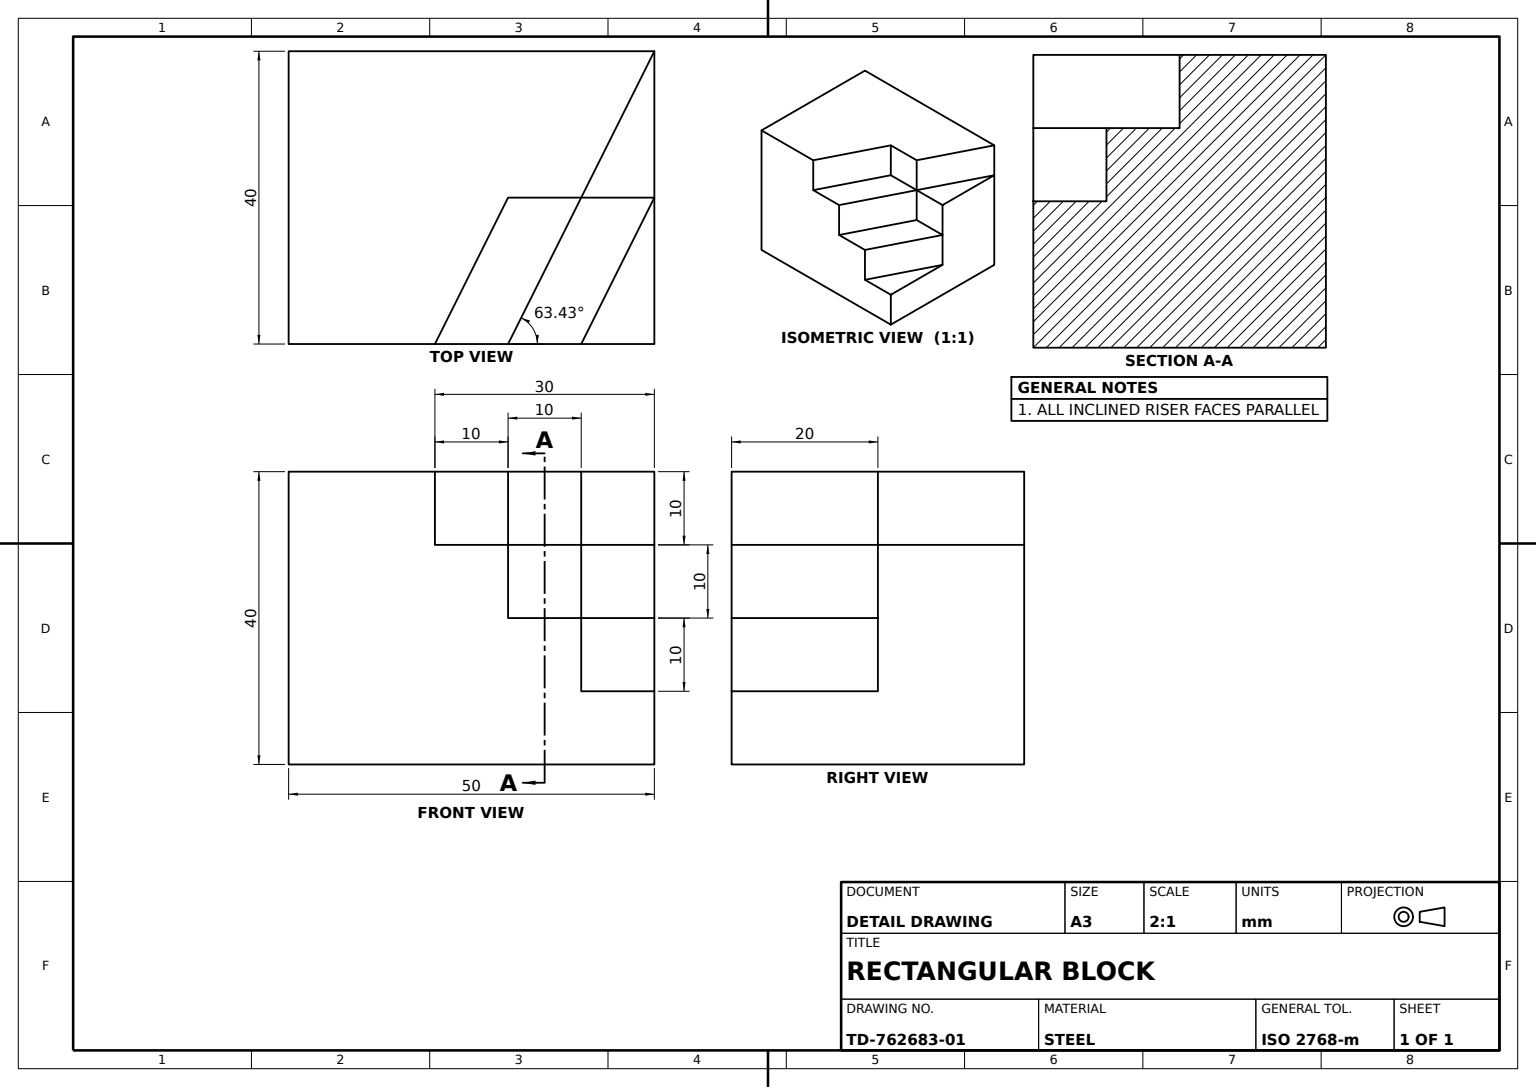
SolidWorks part; units mm, degrees
material "Plain Carbon Steel"
ref_plane "Front Plane" through (0, 0, 0) normal (0, 0, 1) x (1, 0, 0)
ref_plane "Top Plane" through (0, 0, 0) normal (0, 1, 0) x (1, 0, 0)
ref_plane "Right Plane" through (0, 0, 0) normal (1, 0, 0) x (0, 0, -1)
sketch "Base Block Profile" plane through (0, 0, 0) normal (0, 1, 0) x (1, 0, 0)
  line L1 (25, -20) -> (-25, -20)
  line L2 (25, -20) -> (25, 20)
  line L3 (25, 20) -> (-25, 20)
  line L4 (-25, -20) -> (-25, 20)
  line L5 (25, -20) -> (-25, 20) construction
  line L6 (25, 20) -> (-25, -20) construction
  point P0 (0, 0)
  dimension "D1" = 50
  dimension "D2" = 40
extrude "Base Block 50x40x40" add sketch "Base Block Profile" along normal mid plane 40
sketch "Step Cut 1 Profile" plane through (0, 20, 0) normal (0, 1, 0) x (1, 0, 0)
  line L0 (15, 0) -> (5, 0)
  line L1 (-25, 20) -> (-25, -20) construction
  line L2 (5, 0) -> (-5, -20)
  line L3 (-25, -20) -> (25, -20) construction
  line L5 (25, 20) -> (15, 0)
  line L6 (25, -20) -> (25, 20) construction
  line L7 (25, -20) -> (25, 20)
  line L8 (-25, -20) -> (25, -20)
  line M3 (-25, -20) -> (25, -20)
  line M4 (25, -20) -> (25, 20)
  dimension "D1" = 30
  dimension "D2" = 20
  dimension "D3" = 40
extrude "Step Cut 1" cut sketch "Step Cut 1 Profile" against normal blind 10 contours L5 L0 L2 M4 M3
sketch "Step Cut 2 Profile" plane through (0, 10, 0) normal (0, 1, 0) x (1, 0, 0)
  line L0 (15, 0) -> (5, -20)
  line L1 (-5, -20) -> (25, -20) construction
  line L2 (15, 0) -> (25, 0)
  line L3 (25, -20) -> (25, 20) construction
  line L5 (-5, -20) -> (25, -20)
  line L6 (5, -20) -> (25, -20)
  line M2 (25, -20) -> (25, 20)
  line M6 (-5, -20) -> (25, -20)
  dimension "D1" = 10
extrude "Step Cut 2" cut sketch "Step Cut 2 Profile" against normal blind 10 contours L2 L0 M6 M2
sketch "Step Cut 3 Profile" plane through (0, 0, 0) normal (0, 1, 0) x (1, 0, 0)
  line L0 (25, 0) -> (15, -20)
  line L1 (5, -20) -> (25, -20) construction
  line L2 (25, -20) -> (25, 0) construction
  line L3 (25, -20) -> (25, 0)
  line L4 (5, -20) -> (25, -20)
  line M3 (5, -20) -> (25, -20)
  line M4 (25, -20) -> (25, 0)
  dimension "D1" = 10
extrude "Step Cut 3" cut sketch "Step Cut 3 Profile" against normal blind 10 contours L0 M4 M3
